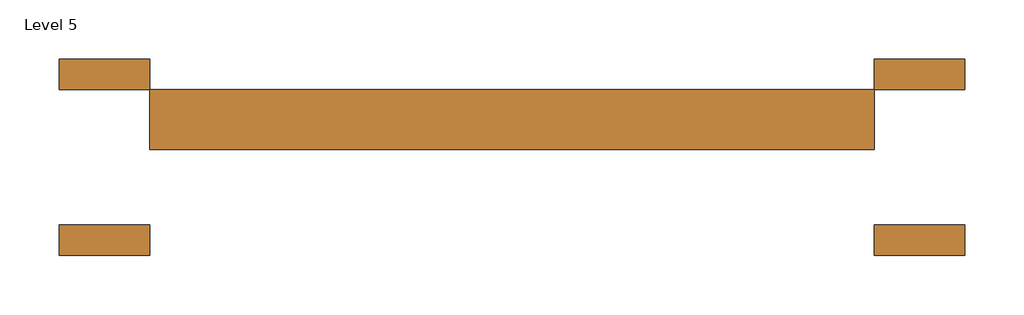
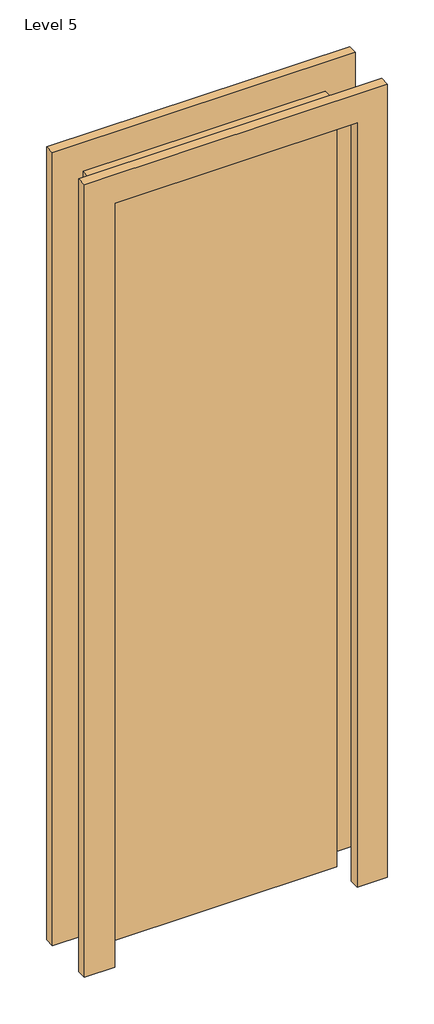
# One storey: 1 door.
"""IFC4 building model written with IfcOpenShell, lengths in millimetres."""

from ifc_helpers import new_model, si_unit, origin, place, context, project, spatial, transform, mapped, element, save
from components import single_flush_bathroom_door_2_x_7_d2bb450e

model = new_model("IFC4")

# Units and contexts
model_context = context("Model", 3, world=origin())
ifc_project = project(units=[si_unit("LENGTHUNIT", "METRE", prefix="MILLI")], contexts=[model_context])

# Site, building, storey
site = spatial("IfcSite", under=ifc_project)
building = spatial("IfcBuilding", under=site)
storey = spatial("IfcBuildingStorey", under=building, Name="Level 5", Elevation=3657.6)

# Door
placement = place(None, origin())
single_flush_bathroom_door_2_x_7_shape = single_flush_bathroom_door_2_x_7_d2bb450e(model_context)
element("IfcDoor", 1, ObjectType="Single-Flush : BATHROOM DOOR 2' X 7'", at=placement, inside=storey, context=model_context, shape_type="MappedRepresentation", body=[
    mapped(single_flush_bathroom_door_2_x_7_shape, transform((-12487.2729553, -872.2535687, 3657.6), x_axis=(1.0, 0.0, 0.0), y_axis=(0.0, 1.0, 0.0), z_axis=(0.0, 0.0, 1.0))),
])

save(model, "model.ifc")

# Revit data of these elements
# Type "Single-Flush : BATHROOM DOOR 2' X 7'"
#   Type Mark = "11"
#   Construction Type Id = "MDOOR"
#   Assembly Code = "C1020"
#   Analytic Construction = "Metal"
#   Thickness = 0' - 2"
#   Heat Transfer Coefficient (U) = 0.651978 BTU/(h·ft²·°F)
#   Height = 6' - 8"
#   Trim Projection Ext = 0' - 1"
#   Trim Projection Int = 0' - 1"
#   Trim Width = 0' - 3"
#   Width = 2' - 0"
#   Define Thermal Properties by = 1
#   Door Material = Door - Panel
#   Frame Material = Door - Frame
#   Visual Light Transmittance = 0
#   Solar Heat Gain Coefficient = 0
#   Function = (empty or 0)
#   Wall Closure = (empty or 0)
# Element 1 (IfcDoor, "Single-Flush : BATHROOM DOOR 2' X 7'")
#   Phase Created = New Construction
#   Materials on its faces: "Door - Frame", "Door - Panel"
# Materials
#   "Door - Panel": class "Wood", colour RGB 210 159 95, transparency 0, Cost = 0
#   "Door - Frame": colour RGB 118 70 51, transparency 0, Cost = 0
